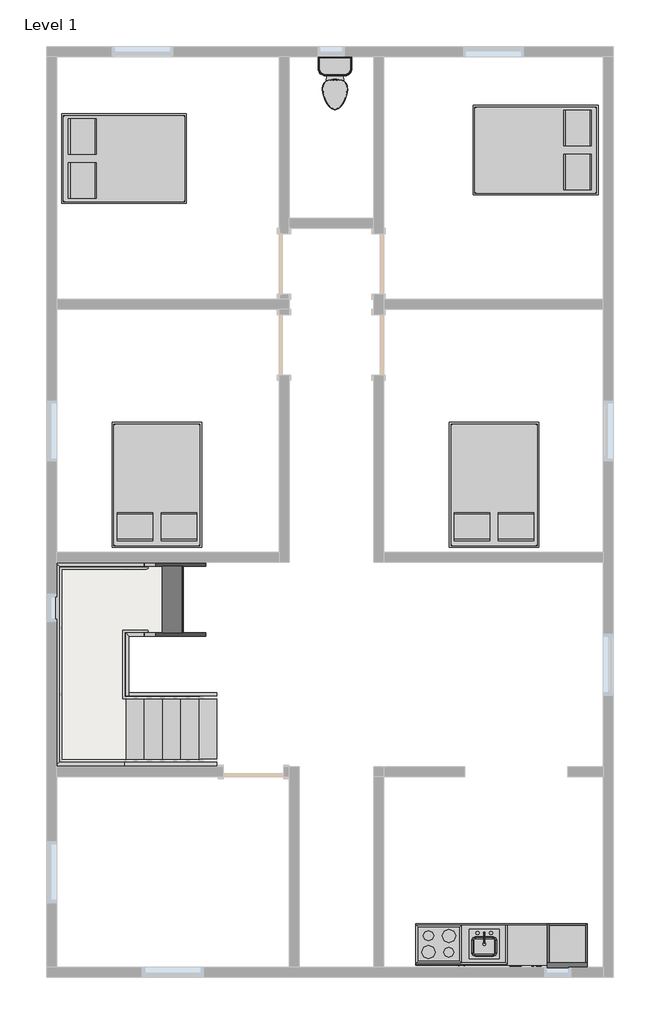
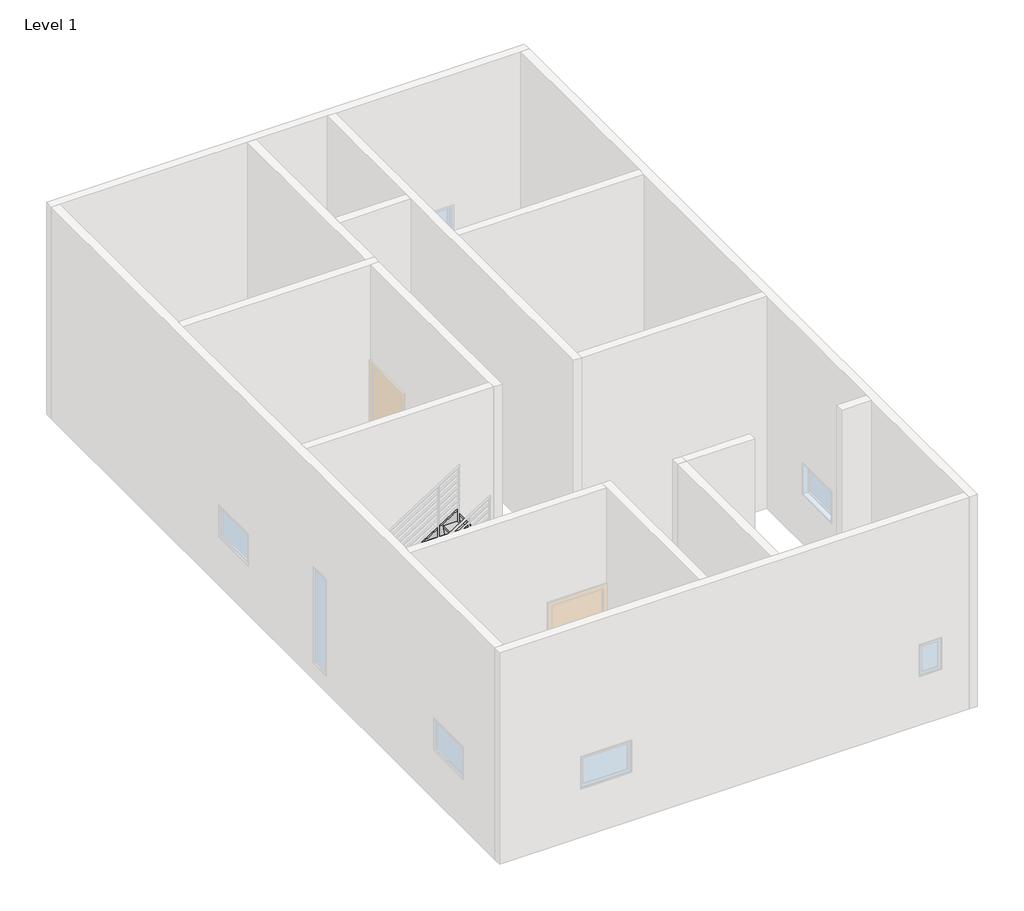
# One storey, part 4 of 4: 9 members, 5 furniture elements, 4 proxies, 2 flow terminals, 2 stair flights, 1 slab.
"""IFC4 building model written with IfcOpenShell, lengths in millimetres."""

from ifc_helpers import new_model, si_unit, frame, origin, place, context, project, spatial, polyline, outline, extrude, faceted_brep, transform, mapped, element, save
from components import m_cook_top_4_unit2_0615_x_500mm_249f3515, m_dishwasher_610_x_610_x_875mm_54ecfc4c, m_kitchenette_medium_1372mm_e05c6bec, m_refrigerator_600_x_660mm_a466bf94, m_sink_kitchen_island_450_x_450mm_f969cf2d, m_toilet_domestic_3d_m_toilet_domestic_3d_5cb52bd4, m_toilet_domestic_3d_m_toilet_domestic_3d_183bbd19, m_bed_box_1346_x_1880mm_double_b32eb57e, m_counter_top_w_sink_hole_600mm_depth_0a237b63, non_monolithic_landing_d31418c5, stair_flight_50mm_tread_25mm_nosing_13mm_riser_f2c6acf0, stair_flight_50mm_tread_25mm_nosing_13mm_riser_f72ebc14

model = new_model("IFC4")

# Units and contexts
model_context = context("Model", 3, world=origin())
ifc_project = project(units=[si_unit("LENGTHUNIT", "METRE", prefix="MILLI")], contexts=[model_context])

# Site, building, storey
site = spatial("IfcSite", under=ifc_project)
building = spatial("IfcBuilding", under=site)
storey = spatial("IfcBuildingStorey", under=building, Name="Level 1", Elevation=0.0)

# Proxies
placement = place(None, origin())
m_cook_top_4_unit2_0615_x_500mm_shape = m_cook_top_4_unit2_0615_x_500mm_249f3515(model_context)
element("IfcBuildingElementProxy", 1, Name="M_Cook Top-4 Unit2 : 0615 x 500mm", ObjectType="M_Cook Top-4 Unit2 : 0615 x 500mm", at=placement, inside=storey, context=model_context, shape_type="MappedRepresentation", body=[
    mapped(m_cook_top_4_unit2_0615_x_500mm_shape, transform((-7246.9381184, -1887.6472617, 0.0), x_axis=(1.0, 0.0, 0.0), y_axis=(0.0, 1.0, 0.0), z_axis=(0.0, 0.0, 1.0))),
])
m_dishwasher_610_x_610_x_875mm_shape = m_dishwasher_610_x_610_x_875mm_54ecfc4c(model_context)
element("IfcBuildingElementProxy", 2, Name="M_Dishwasher : 610 x 610 x 875mm", ObjectType="M_Dishwasher : 610 x 610 x 875mm", at=placement, inside=storey, context=model_context, shape_type="MappedRepresentation", body=[
    mapped(m_dishwasher_610_x_610_x_875mm_shape, transform((-6297.4555869, -2154.2968265, 0.0), x_axis=(1.0, 0.0, 0.0), y_axis=(0.0, 1.0, 0.0), z_axis=(0.0, 0.0, 1.0))),
])
m_kitchenette_medium_1372mm_shape = m_kitchenette_medium_1372mm_e05c6bec(model_context)
element("IfcBuildingElementProxy", 3, Name="M_Kitchenette - Medium : 1372mm", ObjectType="M_Kitchenette - Medium : 1372mm", at=placement, inside=storey, context=model_context, shape_type="MappedRepresentation", body=[
    mapped(m_kitchenette_medium_1372mm_shape, transform((-6922.6758233, -1582.6472617, 0.0), x_axis=(1.0, 0.0, 0.0), y_axis=(0.0, 1.0, 0.0), z_axis=(0.0, 0.0, 1.0))),
])
m_refrigerator_600_x_660mm_shape = m_refrigerator_600_x_660mm_a466bf94(model_context)
element("IfcBuildingElementProxy", 4, Name="M_Refrigerator : 600 x 660mm", ObjectType="M_Refrigerator : 600 x 660mm", at=placement, inside=storey, context=model_context, shape_type="MappedRepresentation", body=[
    mapped(m_refrigerator_600_x_660mm_shape, transform((-5256.1369758, -1878.8623519, 0.0), x_axis=(1.0, 0.0, 0.0), y_axis=(0.0, 1.0, 0.0), z_axis=(0.0, 0.0, 1.0))),
])

# Flow terminals
m_sink_kitchen_island_450_x_450mm_shape = m_sink_kitchen_island_450_x_450mm_f969cf2d(model_context)
element("IfcFlowTerminal", 5, ObjectType="M_Sink Kitchen-Island : 450 x 450mm", at=placement, inside=storey, context=model_context, shape_type="MappedRepresentation", body=[
    mapped(m_sink_kitchen_island_450_x_450mm_shape, transform((-6576.627359, -1889.9926628, 0.0), x_axis=(1.0, 0.0, 0.0), y_axis=(0.0, 1.0, 0.0), z_axis=(0.0, 0.0, 1.0))),
])
m_toilet_domestic_3d_m_toilet_domestic_3d_shape = m_toilet_domestic_3d_m_toilet_domestic_3d_5cb52bd4(model_context)
m_toilet_domestic_3d_m_toilet_domestic_3d_2_shape = m_toilet_domestic_3d_m_toilet_domestic_3d_183bbd19(model_context)
element("IfcFlowTerminal", 6, ObjectType="M_Toilet-Domestic-3D : M_Toilet-Domestic-3D", at=placement, inside=storey, context=model_context, shape_type="MappedRepresentation", body=[
    mapped(m_toilet_domestic_3d_m_toilet_domestic_3d_shape, transform((-8808.9941025, 10984.2567109, 0.0), x_axis=(1.0, 0.0, 0.0), y_axis=(0.0, 1.0, 0.0), z_axis=(0.0, 0.0, 1.0))),
    mapped(m_toilet_domestic_3d_m_toilet_domestic_3d_2_shape, transform((-8808.9941025, 10984.2567109, 0.0), x_axis=(1.0, 0.0, 0.0), y_axis=(0.0, 1.0, 0.0), z_axis=(0.0, 0.0, 1.0))),
])

# Furniture
m_bed_box_1346_x_1880mm_double_shape = m_bed_box_1346_x_1880mm_double_b32eb57e(model_context)
element("IfcFurniture", 7, ObjectType="M_Bed-Box : 1346 x 1880mm - Double", at=placement, inside=storey, context=model_context, shape_type="MappedRepresentation", body=[
    mapped(m_bed_box_1346_x_1880mm_double_shape, transform((-12220.3676266, 9603.2002793, 0.0), x_axis=(0.0, 1.0000000000000002, 0.0), y_axis=(-1.0000000000000002, 0.0, 0.0), z_axis=(0.0, 0.0, 1.0))),
])
element("IfcFurniture", 8, ObjectType="M_Bed-Box : 1346 x 1880mm - Double", at=placement, inside=storey, context=model_context, shape_type="MappedRepresentation", body=[
    mapped(m_bed_box_1346_x_1880mm_double_shape, transform((-5551.9086102, 10408.9051973, 0.0), x_axis=(0.0, -1.0, 0.0), y_axis=(1.0, 0.0, 0.0), z_axis=(0.0, 0.0, 1.0))),
])
element("IfcFurniture", 9, ObjectType="M_Bed-Box : 1346 x 1880mm - Double", at=placement, inside=storey, context=model_context, shape_type="MappedRepresentation", body=[
    mapped(m_bed_box_1346_x_1880mm_double_shape, transform((-11151.7856594, 4793.1232301, 0.0), x_axis=(-1.0000000000000004, 0.0, 0.0), y_axis=(0.0, -1.0000000000000004, 0.0), z_axis=(0.0, 0.0, 1.0))),
])
element("IfcFurniture", 10, ObjectType="M_Bed-Box : 1346 x 1880mm - Double", at=placement, inside=storey, context=model_context, shape_type="MappedRepresentation", body=[
    mapped(m_bed_box_1346_x_1880mm_double_shape, transform((-6072.9856594, 4793.1232301, 0.0), x_axis=(-1.0, 0.0, 0.0), y_axis=(0.0, -1.0, 0.0), z_axis=(0.0, 0.0, 1.0))),
])
m_counter_top_w_sink_hole_600mm_depth_shape = m_counter_top_w_sink_hole_600mm_depth_0a237b63(model_context)
element("IfcFurniture", 11, ObjectType="M_Counter Top w Sink Hole : 600mm Depth", at=placement, inside=storey, context=model_context, shape_type="MappedRepresentation", body=[
    mapped(m_counter_top_w_sink_hole_600mm_depth_shape, transform((-6389.4758233, -1582.6472617, 0.0), x_axis=(1.0, 0.0, 0.0), y_axis=(0.0, 1.0, 0.0), z_axis=(0.0, 0.0, 1.0))),
])

# Members
element("IfcMember", 12, ObjectType="Stringer - 50mm Width", at=placement, inside=storey, context=model_context, shape_type="SweptSolid", body=[
    extrude(outline(polyline([(0.0, -10589.1151057), (215.089535, -10589.1151057), (1090.8719878, -11973.9461092), (690.8719878, -12089.8151693), (0.0, -10997.3738385), (0.0, -10589.1151057)])), frame((0.0, 797.8798105, 0.0), z_axis=(0.0, 1.0, 0.0), x_axis=(0.0, 0.0, 1.0)), (0.0, 0.0, 1.0), 50.0),
])
element("IfcMember", 13, ObjectType="Stringer - 50mm Width", at=placement, inside=storey, context=model_context, shape_type="SweptSolid", body=[
    extrude(outline(polyline([(0.0, -10589.1151057), (215.089535, -10589.1151057), (1053.034199, -11914.1151057), (579.7573231, -11914.1151057), (0.0, -10997.3738385), (0.0, -10589.1151057)])), frame((0.0, 1847.9055917, 0.0), z_axis=(0.0, 1.0, 0.0), x_axis=(0.0, 0.0, 1.0)), (0.0, 0.0, 1.0), 50.0),
])
element("IfcMember", 14, ObjectType="Stringer - 50mm Width", at=placement, inside=storey, context=model_context, shape_type="SweptSolid", body=[
    extrude(outline(polyline([(1090.8719878, -11679.2841022), (690.8719878, -11563.4150421), (1480.9430939, -10314.1151057), (1954.2199698, -10314.1151057), (1090.8719878, -11679.2841022)])), frame((0.0, 3800.1656289, 0.0), z_axis=(0.0, 1.0, 0.0), x_axis=(0.0, 0.0, 1.0)), (0.0, 0.0, 1.0), 50.0),
])
element("IfcMember", 15, ObjectType="Stringer - 50mm Width", at=placement, inside=storey, context=model_context, shape_type="SweptSolid", body=[
    extrude(outline(polyline([(1090.8719878, -11679.2841022), (690.8719878, -11563.4150421), (1480.9430939, -10314.1151057), (1954.2199698, -10314.1151057), (1090.8719878, -11679.2841022)])), frame((0.0, 2750.1398477, 0.0), z_axis=(0.0, 1.0, 0.0), x_axis=(0.0, 0.0, 1.0)), (0.0, 0.0, 1.0), 50.0),
])
element("IfcMember", 16, ObjectType="Stringer - 50mm Width", at=placement, inside=storey, context=model_context, shape_type="Brep", body=[
    faceted_brep([(-11679.2841022, 3800.1656289, 1090.8719878), (-11679.2841022, 3850.1656289, 1090.8719878), (-13014.140887, 3850.1656289, 1090.8719878), (-12964.140887, 3800.1656289, 1090.8719878), (-11563.4150421, 3800.1656289, 690.8719878), (-12964.140887, 3800.1656289, 690.8719878), (-11563.4150421, 3850.1656289, 690.8719878), (-13014.140887, 3850.1656289, 690.8719878)], [[[0, 1, 2, 3]], [[4, 0, 3, 5]], [[6, 4, 5, 7]], [[1, 6, 7, 2]], [[1, 0, 4, 6]], [[2, 7, 5, 3]]]),
])
element("IfcMember", 17, ObjectType="Stringer - 50mm Width", at=placement, inside=storey, context=model_context, shape_type="SweptSolid", body=[
    extrude(outline(polyline([(-13014.140887, 3850.1656289), (-12964.140887, 3800.1656289), (-12964.140887, 847.8798105), (-13014.140887, 797.8798105), (-13014.140887, 3850.1656289)])), frame((0.0, 0.0, 690.8719878), z_axis=(0.0, 0.0, 1.0), x_axis=(1.0, 0.0, 0.0)), (0.0, 0.0, 1.0), 400.0),
])
element("IfcMember", 18, ObjectType="Stringer - 50mm Width", at=placement, inside=storey, context=model_context, shape_type="Brep", body=[
    faceted_brep([(-12964.140887, 847.8798105, 1090.8719878), (-13014.140887, 797.8798105, 1090.8719878), (-11973.9461092, 797.8798105, 1090.8719878), (-11973.9461092, 847.8798105, 1090.8719878), (-12964.140887, 847.8798105, 690.8719878), (-12089.8151693, 847.8798105, 690.8719878), (-13014.140887, 797.8798105, 690.8719878), (-12089.8151693, 797.8798105, 690.8719878)], [[[0, 1, 2, 3]], [[4, 0, 3, 5]], [[6, 4, 5, 7]], [[1, 6, 7, 2]], [[1, 0, 4, 6]], [[2, 7, 5, 3]]]),
])
element("IfcMember", 19, ObjectType="Stringer - 50mm Width", at=placement, inside=storey, context=model_context, shape_type="SweptSolid", body=[
    extrude(outline(polyline([(-11914.1151057, 1847.9055917), (-11964.1151057, 1847.9055917), (-11964.1151057, 2800.1398477), (-11914.1151057, 2750.1398477), (-11914.1151057, 1847.9055917)])), frame((0.0, 0.0, 690.8719878), z_axis=(0.0, 0.0, 1.0), x_axis=(1.0, 0.0, 0.0)), (0.0, 0.0, 1.0), 400.0),
])
element("IfcMember", 20, ObjectType="Stringer - 50mm Width", at=placement, inside=storey, context=model_context, shape_type="Brep", body=[
    faceted_brep([(-11964.1151057, 2800.1398477, 1090.8719878), (-11914.1151057, 2750.1398477, 1090.8719878), (-11679.2841022, 2750.1398477, 1090.8719878), (-11679.2841022, 2800.1398477, 1090.8719878), (-11964.1151057, 2800.1398477, 690.8719878), (-11563.4150421, 2800.1398477, 690.8719878), (-11914.1151057, 2750.1398477, 690.8719878), (-11563.4150421, 2750.1398477, 690.8719878)], [[[0, 1, 2, 3]], [[4, 0, 3, 5]], [[6, 4, 5, 7]], [[1, 6, 7, 2]], [[1, 0, 4, 6]], [[2, 7, 5, 3]]]),
])

# Slab
non_monolithic_landing_shape = non_monolithic_landing_d31418c5(model_context)
element("IfcSlab", 21, ObjectType="Non-Monolithic Landing", at=placement, inside=storey, context=model_context, shape_type="MappedRepresentation", body=[
    mapped(non_monolithic_landing_shape, transform((0.0, 0.0, 0.0), x_axis=(1.0, 0.0, 0.0), y_axis=(0.0, 1.0, 0.0), z_axis=(0.0, 0.0, 1.0))),
])

# Stair flights
stair_flight_50mm_tread_25mm_nosing_13mm_riser_shape = stair_flight_50mm_tread_25mm_nosing_13mm_riser_f2c6acf0(model_context)
element("IfcStairFlight", 22, ObjectType="50mm Tread 25mm Nosing 13mm Riser", at=placement, inside=storey, context=model_context, shape_type="MappedRepresentation", body=[
    mapped(stair_flight_50mm_tread_25mm_nosing_13mm_riser_shape, transform((0.0, 0.0, 0.0), x_axis=(1.0, 0.0, 0.0), y_axis=(0.0, 1.0, 0.0), z_axis=(0.0, 0.0, 1.0))),
])
stair_flight_50mm_tread_25mm_nosing_13mm_riser_2_shape = stair_flight_50mm_tread_25mm_nosing_13mm_riser_f72ebc14(model_context)
element("IfcStairFlight", 23, ObjectType="50mm Tread 25mm Nosing 13mm Riser", at=placement, inside=storey, context=model_context, shape_type="MappedRepresentation", body=[
    mapped(stair_flight_50mm_tread_25mm_nosing_13mm_riser_2_shape, transform((0.0, 0.0, 0.0), x_axis=(1.0, 0.0, 0.0), y_axis=(0.0, 1.0, 0.0), z_axis=(0.0, 0.0, 1.0))),
])

save(model, "model.ifc")

# Revit data of these elements
# Type "M_Cook Top-4 Unit2 : 0615 x 500mm"
#   Depth = 500 mm
#   Width = 615 mm
#   Burner Material = Steel, Chrome Plated
#   Cooktop Material = Steel, Polished
#   Default Elevation = 0
#   Assembly Code = ""
# Type "M_Dishwasher : 610 x 610 x 875mm"
#   Label = "DW"
#   Depth = 610 mm
#   Height = 875 mm
#   Width = 610 mm
#   Dishwasher Material = Steel, Paint Finish, Ivory, Glossy
#   Panel Face Material = Plastic, Opaque Black
#   Default Elevation = 0
# Type "M_Kitchenette - Medium : 1372mm"
#   Counter Length = 1980 mm
#   Cabinet Width = 1372 mm
#   Cabinet Height = 900 mm
#   Cabinet Depth = 610 mm
#   Toe Depth = 35 mm
#   Toe Height = 100 mm
#   Cabinet Material = Cabinets
#   Door/Drawer Material = Cabinets
#   Handle Material = Cabinets - Handles
#   Default Elevation = 0
# Type "M_Refrigerator : 600 x 660mm"
#   Label = "REF."
#   Depth = 660 mm
#   Height = 1830 mm
#   Width = 600 mm
#   Material = Steel, Paint Finish, Ivory, Matte
#   Description = (empty or 0)
#   Default Elevation = 0
# Type "M_Sink Kitchen-Island : 450 x 450mm"
#   Counter Height [instance default] = 900 mm
#   Depth = 450 mm
#   Width = 450 mm
#   Fixture Material = Steel, Polished
#   Sink Material = Steel, Polished
#   Default Elevation = 0
# Type "M_Toilet-Domestic-3D : M_Toilet-Domestic-3D"
#   Bowl/Basin Material = Porcelain, Linen
#   Seat Material = Laminate, Linen, Matte
#   Default Elevation = 0
# Type "M_Bed-Box : 1346 x 1880mm - Double"
#   Length = 1880 mm
#   Width = 1346 mm
#   Frame Material = Birch
#   Mattress Material = Linen, White
#   Default Elevation = 0
# Type "M_Counter Top w Sink Hole : 600mm Depth"
#   Counter Thickness = 40 mm
#   Depth = 625 mm
#   Height = 900 mm
#   Length [instance default] = 2500 mm
#   Sink Location [instance default] = 1200 mm
#   Sink Location To Wall [instance default] = 100 mm
#   Sink Opening Depth [instance default] = 378 mm
#   Sink Opening Width [instance default] = 587 mm
#   Counter Top Material = none
#   Default Elevation = 0
# Element 1 (IfcBuildingElementProxy, "M_Cook Top-4 Unit2 : 0615 x 500mm")
#   Phase Created = New Construction
#   Materials on its faces: "Steel, Polished", "Steel, Chrome Plated"
# Element 2 (IfcBuildingElementProxy, "M_Dishwasher : 610 x 610 x 875mm")
#   Phase Created = New Construction
#   Materials on its faces: "Steel, Paint Finish, Ivory, Glossy", "Plastic, Opaque Black"
# Element 3 (IfcBuildingElementProxy, "M_Kitchenette - Medium : 1372mm")
#   Phase Created = New Construction
#   Materials on its faces: "Cabinets", "Cabinets - Handles"
# Element 4 (IfcBuildingElementProxy, "M_Refrigerator : 600 x 660mm")
#   Phase Created = New Construction
#   Materials on its faces: "Steel, Paint Finish, Ivory, Matte", "Steel, Chrome Plated"
# Element 5 (IfcFlowTerminal, "M_Sink Kitchen-Island : 450 x 450mm")
#   Mark = "1"
#   Counter Height = 900 mm
#   Phase Created = New Construction
#   Materials on its faces: "Steel, Polished"
# Element 6 (IfcFlowTerminal, "M_Toilet-Domestic-3D : M_Toilet-Domestic-3D")
#   Mark = "2"
#   Phase Created = New Construction
#   Materials on its faces: "Porcelain, Linen", "Laminate, Linen, Matte"
# Elements 7, 8, 9, 10 (IfcFurniture, "M_Bed-Box : 1346 x 1880mm - Double")
#   Phase Created = New Construction
#   Materials on its faces: "Birch", "Linen, White"
# Element 11 (IfcFurniture, "M_Counter Top w Sink Hole : 600mm Depth")
#   Sink Opening Width = 400 mm
#   Sink Opening Depth = 350 mm
#   Sink Location To Wall = 160 mm
#   Sink Location = 1025 mm
#   Length = 1980 mm
#   Phase Created = New Construction
#   Materials on its faces: "Counter Top"
# Elements 12, 13, 14, 15, 16, 17, 18, 19, 20 (IfcMember, "Stringer - 50mm Width")
#   Phase Created = New Construction
# Element 21 (IfcSlab, "Non-Monolithic Landing")
#   Phase Created = New Construction
# Elements 22, 23 (IfcStairFlight, "50mm Tread 25mm Nosing 13mm Riser")
#   Phase Created = New Construction
# Materials
#   "Steel, Chrome Plated": class "Metal", colour RGB 244 244 244, transparency 0, Description = "Chromiuim plated steel", Cost = 0
#   "Steel, Polished": class "Metal", colour RGB 57 57 57, transparency 0, Description = "Polished steel", Cost = 0
#   "Steel, Paint Finish, Ivory, Glossy": class "Metal", colour RGB 247 247 239, transparency 0, Description = "Steel, paint finish, ivory, glossy", Cost = 0
#   "Plastic, Opaque Black": class "Plastic", colour RGB 0 0 0, transparency 0.7, Description = "Plastic, generic, opaque black", Cost = 0
#   "Cabinets": colour RGB 249 249 249, transparency 0
#   "Cabinets - Handles": class "Metal", colour RGB 57 57 57, transparency 0
#   "Steel, Paint Finish, Ivory, Matte": class "Metal", colour RGB 247 247 239, transparency 0, Description = "Steel, paint finish, ivory, matte", Cost = 0
#   "Porcelain, Linen": class "Ceramic", colour RGB 249 239 230, transparency 0, Description = "Porcelain, linen", Cost = 0
#   "Laminate, Linen, Matte": class "Plastic", colour RGB 249 239 230, transparency 0, Description = "Plastic Laminate - Linen, Matte", Cost = 0
#   "Birch": class "Wood", colour RGB 224 178 126, transparency 0, Description = "Betula Alleghaniensis", Cost = 0
#   "Linen, White": class "Textile", colour RGB 247 247 239, transparency 0, Description = "Linen, white", Cost = 0
#   "Counter Top": class "Wood", colour RGB 226 177 128, transparency 0
